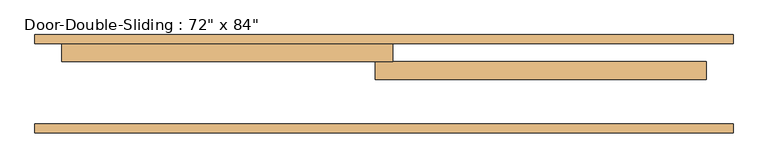
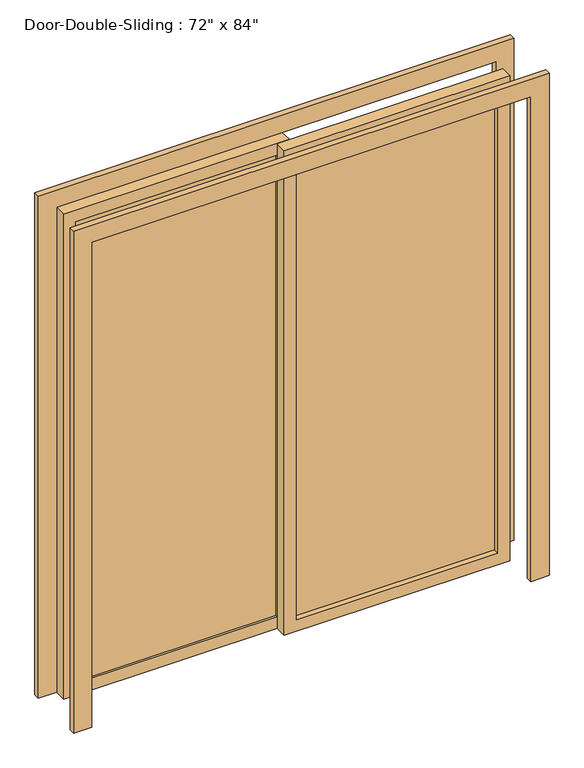
"""IFC4 building model written with IfcOpenShell, lengths in millimetres: door geometry."""

from ifc_helpers import new_model, si_unit, frame, origin, place, context, project, spatial, polyline, outline, extrude, source, transform, mapped, element, save


def door_d4d75d1e(model_context):
    return source(origin(), model_context, "Body", "SweptSolid", [
        extrude(outline(polyline([(0.0, 990.6), (2209.8, 990.6), (2209.8, -990.6), (0.0, -990.6), (0.0, -914.4), (2133.6, -914.4), (2133.6, 914.4), (0.0, 914.4), (0.0, 990.6)])), frame((0.0, 241.3, 0.0), z_axis=(0.0, 1.0, 0.0), x_axis=(0.0, 0.0, 1.0)), (0.0, 0.0, 1.0), 25.4),
        extrude(outline(polyline([(0.0, -990.6), (0.0, -914.4), (2133.6, -914.4), (2133.6, 914.4), (0.0, 914.4), (0.0, 990.6), (2209.8, 990.6), (2209.8, -990.6), (0.0, -990.6)])), frame((0.0, -12.7, 0.0), z_axis=(0.0, 1.0, 0.0), x_axis=(0.0, 0.0, 1.0)), (0.0, 0.0, 1.0), 25.4),
        extrude(outline(polyline([(2133.6, 25.4), (2133.6, -914.4), (0.0, -914.4), (0.0, 25.4), (2133.6, 25.4)]), holes=[polyline([(2082.8, -25.4), (50.8, -25.4), (50.8, -863.6), (2082.8, -863.6), (2082.8, -25.4)])]), frame((0.0, 190.5, 0.0), z_axis=(0.0, 1.0, 0.0), x_axis=(0.0, 0.0, 1.0)), (0.0, 0.0, 1.0), 50.8),
        extrude(outline(polyline([(2133.6, -25.4), (0.0, -25.4), (0.0, 914.4), (2133.6, 914.4), (2133.6, -25.4)]), holes=[polyline([(2082.8, 25.4), (2082.8, 863.6), (50.8, 863.6), (50.8, 25.4), (2082.8, 25.4)])]), frame((0.0, 139.7, 0.0), z_axis=(0.0, 1.0, 0.0), x_axis=(0.0, 0.0, 1.0)), (0.0, 0.0, 1.0), 50.8),
        extrude(outline(polyline([(-25.4, 200.025), (-863.6, 200.025), (-863.6, 206.375), (-25.4, 206.375), (-25.4, 200.025)])), frame((0.0, 0.0, 50.8), z_axis=(0.0, 0.0, 1.0), x_axis=(1.0, 0.0, 0.0)), (0.0, 0.0, 1.0), 2032.0),
        extrude(outline(polyline([(25.4, 168.275), (863.6, 168.275), (863.6, 161.925), (25.4, 161.925), (25.4, 168.275)])), frame((0.0, 0.0, 50.8), z_axis=(0.0, 0.0, 1.0), x_axis=(1.0, 0.0, 0.0)), (0.0, 0.0, 1.0), 2032.0),
    ])


if __name__ == "__main__":
    model = new_model("IFC4")
    model_context = context("Model", 3, world=origin())
    ifc_project = project(units=[si_unit("LENGTHUNIT", "METRE", prefix="MILLI")], contexts=[model_context])
    site = spatial("IfcSite", under=ifc_project)
    building = spatial("IfcBuilding", under=site)
    placement = place(None, origin())
    door_shape = door_d4d75d1e(model_context)
    element("IfcDoor", 1, ObjectType="Door-Double-Sliding : 72\" x 84\"", at=placement, inside=building, context=model_context, shape_type="MappedRepresentation", body=[
        mapped(door_shape, transform((0.0, 0.0, 0.0), x_axis=(1.0, 0.0, 0.0), y_axis=(0.0, 1.0, 0.0), z_axis=(0.0, 0.0, 1.0))),
    ])
    save(model, "model.ifc")

# Revit data of these elements
# Type "Door-Double-Sliding : 72\" x 84\""
#   Type Mark = "14"
#   Construction Type Id = "opn-d45"
#   Assembly Code = "C1020"
#   Analytic Construction = "Wood frame, double glass door "
#   Thickness = 0' - 2"
#   Thermal Resistance (R) = 1.8150 (h·ft²·°F)/BTU
#   Heat Transfer Coefficient (U) = 0.5510 BTU/(h·ft²·°F)
#   Height = 7' - 0"
#   Rail Width = 0' - 2"
#   Stiles = 0' - 2"
#   Trim Projection Ext = 0' - 1"
#   Trim Projection Int = 0' - 1"
#   Trim Width = 0' - 3"
#   Width = 6' - 0"
#   Define Thermal Properties by = 1
#   Glazing = Glass
#   Panel Material = Wood - Birch - Solid Stained Light Low Gloss
#   Trim Material = Paint - Sienna
#   Visual Light Transmittance = 0
#   Solar Heat Gain Coefficient = 0
#   Function = (empty or 0)
#   Wall Closure = (empty or 0)
# Element 1 (IfcDoor, "Door-Double-Sliding : 72\" x 84\"")
#   Materials on its faces: "Paint - Sienna", "Wood - Birch - Solid Stained Light Low Gloss", "Glass"
# Materials
#   "Glass": class "Glass", colour RGB 0 128 192, transparency 0.75, Description = "Soda Lime Glass", Cost = 0
#   "Wood - Birch - Solid Stained Light Low Gloss": class "Wood", colour RGB 210 159 95, transparency 0, Cost = 0
#   "Paint - Sienna": colour RGB 118 70 51, transparency 0, Cost = 0
